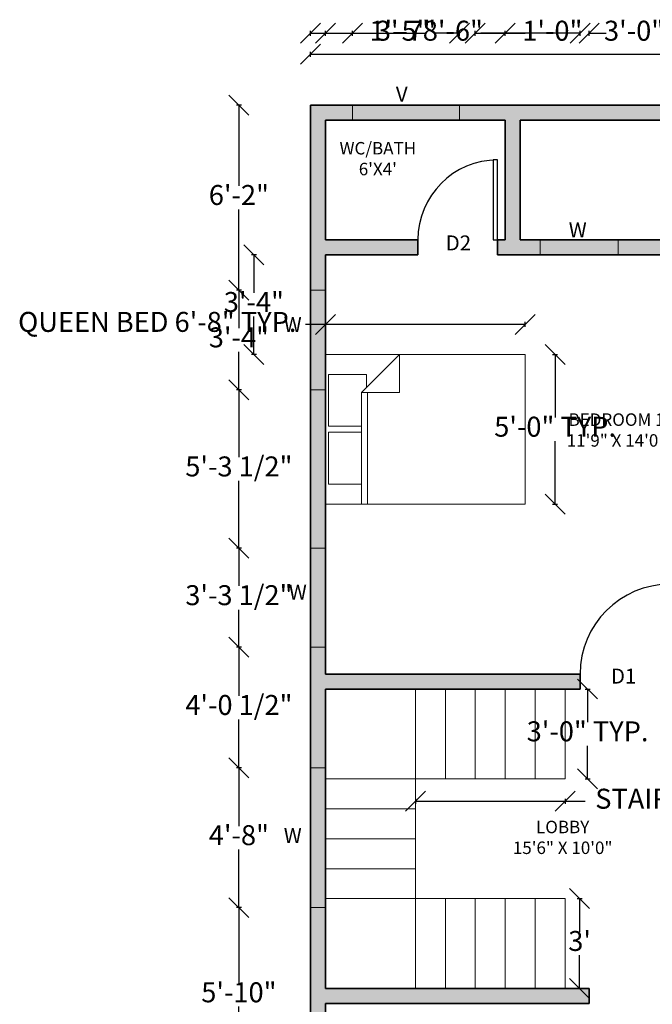
# Model space of a CAD drawing. Units: inches. Extents: x 2247 to 2713, y 588 to 1209.
# Tile 4 of 5: x 2247 to 2501, y 808 to 1202. Entities that reach past the tile are written whole.
import ezdxf

# ---------------------------------------------------------------- set-up
doc = ezdxf.new("R2010")
doc.units = ezdxf.units.IN
for name, color, linetype, lineweight in [('A-ANNO-DIMS', 2, 'Continuous', 18), ('A-ANNO-TEXT', 7, 'Continuous', 18), ('A-AREA-IDEN', 7, 'Continuous', 25), ('A-DOOR', 3, 'Continuous', 25), ('A-FLOR-STRS', 7, 'Continuous', 18), ('A-FURN', 8, 'Continuous', 18), ('A-GLAZ', 4, 'Continuous', 18), ('A-GLAZ-PATT', 7, 'Continuous', 13), ('A-WALL', 7, 'Continuous', 35), ('A-WALL-PATT', 4, 'Continuous', 13)]:
    doc.layers.add(name, color=color, linetype=linetype, lineweight=lineweight)
doc.styles.get("Standard").update_dxf_attribs({"font": 'arial.ttf'})
doc.dimstyles.new('ISO-25', dxfattribs={"dimtxt": 8, "dimasz": 8, "dimexe": 1, "dimexo": 1, "dimtad": 0, "dimtih": 1, "dimtoh": 1, "dimlunit": 3, "dimtxsty": 'Standard', "dimblk": 'OBLIQUE', "dimcen": 2.5, "dimadec": 0, "dimazin": 0, "dimtfac": 1, "dimtmove": 0, "dimatfit": 3, "dimfxl": 1, "dimfxlon": 1, "dimarcsym": 0})

# ---------------------------------------------------------------- blocks, each defined once
blk = doc.blocks.new('*U4')
for p, q in [((0, 0), (0, -6)), ((-36, 0), (-36, -6))]:
    blk.add_line(p, q)
blk.add_lwpolyline([(0, 0), (0, 36), (-1.75, 36), (-1.75, 0)], close=True)
blk.add_arc((0, 0), 36, 90, 180)
blk = doc.blocks.new('*U6')
for p, q in [((0, 0), (0, -6)), ((-32, 0), (-32, -6))]:
    blk.add_line(p, q)
blk.add_lwpolyline([(0, 0), (0, 32), (-1.75, 32), (-1.75, 0)], close=True)
blk.add_arc((0, 0), 32, 90, 180)
blk = doc.blocks.new('Bed - Queen')
for p, q in [((0, -80.00003), (0, 0)), ((0, 0), (59.99999, 0)), ((59.99999, 0), (59.99999, -80.00003)), ((7.99999, -1.2), (28.79998, -1.2)), ((7.99999, -14.4), (7.99999, -1.2)), ((28.79998, -1.2), (28.79998, -14.4)), ((31.19999, -1.2), (51.99999, -1.2)), ((31.19999, -14.4), (31.19999, -1.2)), ((51.99999, -1.2), (51.99999, -16.4)), ((0, -14.4), (44.8, -14.4)), ((59.99999, -29.6), (44.8, -14.4)), ((44.8, -14.4), (44.8, -29.6)), ((44.8, -16.8), (0, -16.8)), ((51.99999, -16.4), (46.79936, -16.4)), ((44.8, -29.6), (59.99999, -29.6)), ((59.99999, -80.00003), (0, -80.00003))]:
    blk.add_line(p, q)
blk = doc.blocks.new('_Oblique')
at = {"color": 0, "linetype": 'ByBlock', "lineweight": -2}
blk.add_line((-0.5, -0.5), (0.5, 0.5), dxfattribs=at)
blk = doc.blocks.new('*D11')
at = {"layer": 'A-ANNO-DIMS', "color": 0, "lineweight": -2, "transparency": 16777216}
for p, q in [((2364.08, 1187.64), (2364.08, 1189.64)), ((2364.08, 1188.64), (2506.59, 1188.64)), ((2664.08, 1188.64), (2521.56, 1188.64)), ((2664.08, 1187.64), (2664.08, 1189.64))]:
    blk.add_line(p, q, dxfattribs=at)
at = {"layer": 'Defpoints', "color": 0, "transparency": 16777216}
for p in [(2664.08, 1188.64), (2364.08, 1168.28), (2664.08, 1168.28)]:
    blk.add_point(p, dxfattribs=at)
at = {"layer": 'A-ANNO-DIMS', "color": 0, "lineweight": -2, "transparency": 16777216, "xscale": 8, "yscale": 8, "zscale": 8, "rotation": 180}
blk.add_blockref('_Oblique', (2364.08, 1188.64), dxfattribs=at)
at = {"layer": 'A-ANNO-DIMS', "color": 0, "lineweight": -2, "transparency": 16777216, "xscale": 8, "yscale": 8, "zscale": 8}
blk.add_blockref('_Oblique', (2664.08, 1188.64), dxfattribs=at)
at = {"layer": 'A-ANNO-DIMS', "color": 0, "transparency": 16777216, "insert": (2514.08, 1188.64), "char_height": 8, "attachment_point": 5}
blk.add_mtext("25'", dxfattribs=at)
blk = doc.blocks.new('*D13')
at = {"layer": 'A-ANNO-DIMS', "color": 0, "lineweight": -2, "transparency": 16777216}
for p, q in [((2470.88, 850.28), (2472.88, 850.28)), ((2471.88, 850.28), (2471.88, 836.99)), ((2471.88, 814.28), (2471.88, 827.57)), ((2470.88, 814.28), (2472.88, 814.28))]:
    blk.add_line(p, q, dxfattribs=at)
at = {"layer": 'Defpoints', "color": 0, "transparency": 16777216}
for p in [(2466.08, 850.28), (2466.08, 814.28), (2471.88, 814.28)]:
    blk.add_point(p, dxfattribs=at)
at = {"layer": 'A-ANNO-DIMS', "color": 0, "lineweight": -2, "transparency": 16777216, "xscale": 8, "yscale": 8, "zscale": 8}
for p, rotation in [((2471.88, 850.28), 90), ((2471.88, 814.28), 270)]:
    blk.add_blockref('_Oblique', p, dxfattribs=dict(at, rotation=rotation))
at = {"layer": 'A-ANNO-DIMS', "color": 0, "transparency": 16777216, "insert": (2471.88, 832.28), "char_height": 8, "attachment_point": 5}
blk.add_mtext("3'", dxfattribs=at)
blk = doc.blocks.new('STAIR-FLIGHT-36IN-12IN-GOING')
for p, q in [((0, 36), (0, 0)), ((12, 36), (12, 0)), ((24, 36), (24, 0)), ((36, 36), (36, 0)), ((48, 36), (48, 0)), ((60, 36), (60, 0))]:
    blk.add_line(p, q)
blk = doc.blocks.new('*D15')
at = {"layer": 'A-ANNO-DIMS', "color": 0, "lineweight": -2, "transparency": 16777216}
for p, q in [((2370.08, 1079.35), (2370.08, 1081.35)), ((2450.08, 1079.35), (2450.08, 1081.35)), ((2370.08, 1080.35), (2362.08, 1080.35)), ((2450.08, 1080.35), (2370.08, 1080.35))]:
    blk.add_line(p, q, dxfattribs=at)
at = {"layer": 'Defpoints', "color": 0, "transparency": 16777216}
for p in [(2370.08, 1080.35), (2370.08, 1068.35), (2450.08, 1068.35)]:
    blk.add_point(p, dxfattribs=at)
at = {"layer": 'A-ANNO-DIMS', "color": 0, "lineweight": -2, "transparency": 16777216, "xscale": 8, "yscale": 8, "zscale": 8, "rotation": 180}
blk.add_blockref('_Oblique', (2370.08, 1080.35), dxfattribs=at)
at = {"layer": 'A-ANNO-DIMS', "color": 0, "lineweight": -2, "transparency": 16777216, "xscale": 8, "yscale": 8, "zscale": 8}
blk.add_blockref('_Oblique', (2450.08, 1080.35), dxfattribs=at)
at = {"layer": 'A-ANNO-DIMS', "color": 0, "transparency": 16777216, "insert": (2302.61, 1080.35), "char_height": 8, "attachment_point": 5}
blk.add_mtext('QUEEN BED 6\'-8" TYP.', dxfattribs=at)
blk = doc.blocks.new('*D16')
at = {"layer": 'A-ANNO-DIMS', "color": 0, "lineweight": -2, "transparency": 16777216}
for p, q in [((2461.08, 1068.35), (2463.08, 1068.35)), ((2462.08, 1068.35), (2462.08, 1043.06)), ((2462.08, 1008.35), (2462.08, 1033.64)), ((2461.08, 1008.35), (2463.08, 1008.35))]:
    blk.add_line(p, q, dxfattribs=at)
at = {"layer": 'Defpoints', "color": 0, "transparency": 16777216}
for p in [(2450.08, 1068.35), (2462.08, 1068.35), (2450.08, 1008.35)]:
    blk.add_point(p, dxfattribs=at)
at = {"layer": 'A-ANNO-DIMS', "color": 0, "lineweight": -2, "transparency": 16777216, "xscale": 8, "yscale": 8, "zscale": 8}
for p, rotation in [((2462.08, 1068.35), 90), ((2462.08, 1008.35), 270)]:
    blk.add_blockref('_Oblique', p, dxfattribs=dict(at, rotation=rotation))
at = {"layer": 'A-ANNO-DIMS', "color": 0, "transparency": 16777216, "insert": (2462.08, 1038.35), "char_height": 8, "attachment_point": 5}
blk.add_mtext('5\'-0" TYP.', dxfattribs=at)
blk = doc.blocks.new('*D17')
at = {"layer": 'A-ANNO-DIMS', "color": 0, "lineweight": -2, "transparency": 16777216}
for p, q in [((2406.08, 890.28), (2406.08, 888.28)), ((2406.08, 889.28), (2466.08, 889.28)), ((2466.08, 890.28), (2466.08, 888.28)), ((2466.08, 889.28), (2474.08, 889.28))]:
    blk.add_line(p, q, dxfattribs=at)
at = {"layer": 'Defpoints', "color": 0, "transparency": 16777216}
for p in [(2406.08, 898.28), (2466.08, 898.28), (2466.08, 889.28)]:
    blk.add_point(p, dxfattribs=at)
at = {"layer": 'A-ANNO-DIMS', "color": 0, "lineweight": -2, "transparency": 16777216, "xscale": 8, "yscale": 8, "zscale": 8, "rotation": 180}
blk.add_blockref('_Oblique', (2406.08, 889.28), dxfattribs=at)
at = {"layer": 'A-ANNO-DIMS', "color": 0, "lineweight": -2, "transparency": 16777216, "xscale": 8, "yscale": 8, "zscale": 8}
blk.add_blockref('_Oblique', (2466.08, 889.28), dxfattribs=at)
at = {"layer": 'A-ANNO-DIMS', "color": 0, "transparency": 16777216, "insert": (2538.49, 889.28), "char_height": 8, "attachment_point": 5}
blk.add_mtext('STAIR FLIGHT 5\'-0" TYP.', dxfattribs=at)
blk = doc.blocks.new('*D18')
at = {"layer": 'A-ANNO-DIMS', "color": 0, "lineweight": -2, "transparency": 16777216}
for p, q in [((2474.08, 934.28), (2476.08, 934.28)), ((2475.08, 934.28), (2475.08, 920.99)), ((2475.08, 898.28), (2475.08, 911.57)), ((2474.08, 898.28), (2476.08, 898.28))]:
    blk.add_line(p, q, dxfattribs=at)
at = {"layer": 'Defpoints', "color": 0, "transparency": 16777216}
for p in [(2466.08, 934.28), (2475.08, 934.28), (2466.08, 898.28)]:
    blk.add_point(p, dxfattribs=at)
at = {"layer": 'A-ANNO-DIMS', "color": 0, "lineweight": -2, "transparency": 16777216, "xscale": 8, "yscale": 8, "zscale": 8}
for p, rotation in [((2475.08, 934.28), 90), ((2475.08, 898.28), 270)]:
    blk.add_blockref('_Oblique', p, dxfattribs=dict(at, rotation=rotation))
at = {"layer": 'A-ANNO-DIMS', "color": 0, "transparency": 16777216, "insert": (2475.08, 916.28), "char_height": 8, "attachment_point": 5}
blk.add_mtext('3\'-0" TYP.', dxfattribs=at)
blk = doc.blocks.new('*D27')
at = {"layer": 'A-ANNO-DIMS', "color": 0, "lineweight": -2, "transparency": 16777216}
for p, q in [((2407.02, 600.53), (2407.02, 598.53)), ((2439.02, 600.53), (2439.02, 598.53)), ((2407.02, 599.53), (2411.7, 599.53)), ((2439.02, 599.53), (2434.35, 599.53))]:
    blk.add_line(p, q, dxfattribs=at)
at = {"layer": 'Defpoints', "color": 0, "transparency": 16777216}
for p in [(2407.02, 1108.28), (2439.02, 1108.28), (2439.02, 599.53)]:
    blk.add_point(p, dxfattribs=at)
at = {"layer": 'A-ANNO-DIMS', "color": 0, "lineweight": -2, "transparency": 16777216, "xscale": 8, "yscale": 8, "zscale": 8, "rotation": 180}
blk.add_blockref('_Oblique', (2407.02, 599.53), dxfattribs=at)
at = {"layer": 'A-ANNO-DIMS', "color": 0, "lineweight": -2, "transparency": 16777216, "xscale": 8, "yscale": 8, "zscale": 8}
blk.add_blockref('_Oblique', (2439.02, 599.53), dxfattribs=at)
at = {"layer": 'A-ANNO-DIMS', "color": 0, "transparency": 16777216, "insert": (2423.02, 599.53), "char_height": 8, "attachment_point": 5}
blk.add_mtext('2\'-8"', dxfattribs=at)
blk = doc.blocks.new('*D29')
at = {"layer": 'A-ANNO-DIMS', "color": 0, "lineweight": -2, "transparency": 16777216}
for p, q in [((2336.33, 1094.13), (2334.33, 1094.13)), ((2335.33, 1094.13), (2335.33, 1078.86)), ((2335.33, 1054.17), (2335.33, 1069.44)), ((2336.33, 1054.17), (2334.33, 1054.17))]:
    blk.add_line(p, q, dxfattribs=at)
at = {"layer": 'Defpoints', "color": 0, "transparency": 16777216}
for p in [(2335.33, 1094.13), (2364.08, 1094.13), (2364.08, 1054.17)]:
    blk.add_point(p, dxfattribs=at)
at = {"layer": 'A-ANNO-DIMS', "color": 0, "lineweight": -2, "transparency": 16777216, "xscale": 8, "yscale": 8, "zscale": 8}
for p, rotation in [((2335.33, 1094.13), 90), ((2335.33, 1054.17), 270)]:
    blk.add_blockref('_Oblique', p, dxfattribs=dict(at, rotation=rotation))
at = {"layer": 'A-ANNO-DIMS', "color": 0, "transparency": 16777216, "insert": (2335.33, 1074.15), "char_height": 8, "attachment_point": 5}
blk.add_mtext('3\'-4"', dxfattribs=at)
blk = doc.blocks.new('*D30')
at = {"layer": 'A-ANNO-DIMS', "color": 0, "lineweight": -2, "transparency": 16777216}
for p, q in [((2336.33, 990.69), (2334.33, 990.69)), ((2335.33, 990.69), (2335.33, 975.6)), ((2335.33, 950.99), (2335.33, 966.07)), ((2336.33, 950.99), (2334.33, 950.99))]:
    blk.add_line(p, q, dxfattribs=at)
at = {"layer": 'Defpoints', "color": 0, "transparency": 16777216}
for p in [(2335.33, 990.69), (2364.08, 990.69), (2364.08, 950.99)]:
    blk.add_point(p, dxfattribs=at)
at = {"layer": 'A-ANNO-DIMS', "color": 0, "lineweight": -2, "transparency": 16777216, "xscale": 8, "yscale": 8, "zscale": 8}
for p, rotation in [((2335.33, 990.69), 90), ((2335.33, 950.99), 270)]:
    blk.add_blockref('_Oblique', p, dxfattribs=dict(at, rotation=rotation))
at = {"layer": 'A-ANNO-DIMS', "color": 0, "transparency": 16777216, "insert": (2335.33, 970.84), "char_height": 8, "attachment_point": 5}
blk.add_mtext('3\'-3 1/2"', dxfattribs=at)
blk = doc.blocks.new('*D31')
at = {"layer": 'A-ANNO-DIMS', "color": 0, "lineweight": -2, "transparency": 16777216}
for p, q in [((2336.33, 1054.17), (2334.33, 1054.17)), ((2335.33, 1054.17), (2335.33, 1027.19)), ((2335.33, 990.69), (2335.33, 1017.67)), ((2336.33, 990.69), (2334.33, 990.69))]:
    blk.add_line(p, q, dxfattribs=at)
at = {"layer": 'Defpoints', "color": 0, "transparency": 16777216}
for p in [(2335.33, 1054.17), (2364.08, 1054.17), (2364.08, 990.69)]:
    blk.add_point(p, dxfattribs=at)
at = {"layer": 'A-ANNO-DIMS', "color": 0, "lineweight": -2, "transparency": 16777216, "xscale": 8, "yscale": 8, "zscale": 8}
for p, rotation in [((2335.33, 1054.17), 90), ((2335.33, 990.69), 270)]:
    blk.add_blockref('_Oblique', p, dxfattribs=dict(at, rotation=rotation))
at = {"layer": 'A-ANNO-DIMS', "color": 0, "transparency": 16777216, "insert": (2335.33, 1022.43), "char_height": 8, "attachment_point": 5}
blk.add_mtext('5\'-3 1/2"', dxfattribs=at)
blk = doc.blocks.new('*D32')
at = {"layer": 'A-ANNO-DIMS', "color": 0, "lineweight": -2, "transparency": 16777216}
for p, q in [((2336.33, 1168.28), (2334.33, 1168.28)), ((2335.33, 1168.28), (2335.33, 1135.91)), ((2335.33, 1094.13), (2335.33, 1126.49)), ((2336.33, 1094.13), (2334.33, 1094.13))]:
    blk.add_line(p, q, dxfattribs=at)
at = {"layer": 'Defpoints', "color": 0, "transparency": 16777216}
for p in [(2335.33, 1168.28), (2364.08, 1168.28), (2364.08, 1094.13)]:
    blk.add_point(p, dxfattribs=at)
at = {"layer": 'A-ANNO-DIMS', "color": 0, "lineweight": -2, "transparency": 16777216, "xscale": 8, "yscale": 8, "zscale": 8}
for p, rotation in [((2335.33, 1168.28), 90), ((2335.33, 1094.13), 270)]:
    blk.add_blockref('_Oblique', p, dxfattribs=dict(at, rotation=rotation))
at = {"layer": 'A-ANNO-DIMS', "color": 0, "transparency": 16777216, "insert": (2335.33, 1131.2), "char_height": 8, "attachment_point": 5}
blk.add_mtext('6\'-2"', dxfattribs=at)
blk = doc.blocks.new('*D35')
at = {"layer": 'A-ANNO-DIMS', "color": 0, "lineweight": -2, "transparency": 16777216}
for p, q in [((2336.33, 846.66), (2334.33, 846.66)), ((2335.33, 846.66), (2335.33, 816.41)), ((2335.33, 776.75), (2335.33, 806.99)), ((2336.33, 776.75), (2334.33, 776.75))]:
    blk.add_line(p, q, dxfattribs=at)
at = {"layer": 'Defpoints', "color": 0, "transparency": 16777216}
for p in [(2335.33, 846.66), (2364.08, 846.66), (2364.08, 776.75)]:
    blk.add_point(p, dxfattribs=at)
at = {"layer": 'A-ANNO-DIMS', "color": 0, "lineweight": -2, "transparency": 16777216, "xscale": 8, "yscale": 8, "zscale": 8}
for p, rotation in [((2335.33, 846.66), 90), ((2335.33, 776.75), 270)]:
    blk.add_blockref('_Oblique', p, dxfattribs=dict(at, rotation=rotation))
at = {"layer": 'A-ANNO-DIMS', "color": 0, "transparency": 16777216, "insert": (2335.33, 811.7), "char_height": 8, "attachment_point": 5}
blk.add_mtext('5\'-10"', dxfattribs=at)
blk = doc.blocks.new('*D36')
at = {"layer": 'A-ANNO-DIMS', "color": 0, "lineweight": -2, "transparency": 16777216}
for p, q in [((2336.33, 902.69), (2334.33, 902.69)), ((2335.33, 902.69), (2335.33, 879.38)), ((2335.33, 846.66), (2335.33, 869.97)), ((2336.33, 846.66), (2334.33, 846.66))]:
    blk.add_line(p, q, dxfattribs=at)
at = {"layer": 'Defpoints', "color": 0, "transparency": 16777216}
for p in [(2335.33, 902.69), (2364.08, 902.69), (2364.08, 846.66)]:
    blk.add_point(p, dxfattribs=at)
at = {"layer": 'A-ANNO-DIMS', "color": 0, "lineweight": -2, "transparency": 16777216, "xscale": 8, "yscale": 8, "zscale": 8}
for p, rotation in [((2335.33, 902.69), 90), ((2335.33, 846.66), 270)]:
    blk.add_blockref('_Oblique', p, dxfattribs=dict(at, rotation=rotation))
at = {"layer": 'A-ANNO-DIMS', "color": 0, "transparency": 16777216, "insert": (2335.33, 874.67), "char_height": 8, "attachment_point": 5}
blk.add_mtext('4\'-8"', dxfattribs=at)
blk = doc.blocks.new('*D37')
at = {"layer": 'A-ANNO-DIMS', "color": 0, "lineweight": -2, "transparency": 16777216}
for p, q in [((2336.33, 950.99), (2334.33, 950.99)), ((2335.33, 950.99), (2335.33, 931.6)), ((2335.33, 902.69), (2335.33, 922.08)), ((2336.33, 902.69), (2334.33, 902.69))]:
    blk.add_line(p, q, dxfattribs=at)
at = {"layer": 'Defpoints', "color": 0, "transparency": 16777216}
for p in [(2335.33, 950.99), (2364.08, 950.99), (2364.08, 902.69)]:
    blk.add_point(p, dxfattribs=at)
at = {"layer": 'A-ANNO-DIMS', "color": 0, "lineweight": -2, "transparency": 16777216, "xscale": 8, "yscale": 8, "zscale": 8}
for p, rotation in [((2335.33, 950.99), 90), ((2335.33, 902.69), 270)]:
    blk.add_blockref('_Oblique', p, dxfattribs=dict(at, rotation=rotation))
at = {"layer": 'A-ANNO-DIMS', "color": 0, "transparency": 16777216, "insert": (2335.33, 926.84), "char_height": 8, "attachment_point": 5}
blk.add_mtext('4\'-0 1/2"', dxfattribs=at)
blk = doc.blocks.new('*D41')
at = {"layer": 'A-ANNO-DIMS', "color": 0, "lineweight": -2, "transparency": 16777216}
for p, q in [((2380.83, 1196.03), (2380.83, 1198.03)), ((2380.83, 1197.03), (2391.02, 1197.03)), ((2423.72, 1197.03), (2413.53, 1197.03)), ((2423.72, 1196.03), (2423.72, 1198.03))]:
    blk.add_line(p, q, dxfattribs=at)
at = {"layer": 'Defpoints', "color": 0, "transparency": 16777216}
for p in [(2423.72, 1197.03), (2380.83, 1168.28), (2423.72, 1168.28)]:
    blk.add_point(p, dxfattribs=at)
at = {"layer": 'A-ANNO-DIMS', "color": 0, "lineweight": -2, "transparency": 16777216, "xscale": 8, "yscale": 8, "zscale": 8, "rotation": 180}
blk.add_blockref('_Oblique', (2380.83, 1197.03), dxfattribs=at)
at = {"layer": 'A-ANNO-DIMS', "color": 0, "lineweight": -2, "transparency": 16777216, "xscale": 8, "yscale": 8, "zscale": 8}
blk.add_blockref('_Oblique', (2423.72, 1197.03), dxfattribs=at)
at = {"layer": 'A-ANNO-DIMS', "color": 0, "transparency": 16777216, "insert": (2402.27, 1197.03), "char_height": 8, "attachment_point": 5}
blk.add_mtext('3\'-7"', dxfattribs=at)
blk = doc.blocks.new('*D43')
at = {"layer": 'A-ANNO-DIMS', "color": 0, "lineweight": -2, "transparency": 16777216}
for p, q in [((2364.08, 1196.03), (2364.08, 1198.03)), ((2364.08, 1197.03), (2380.83, 1197.03)), ((2380.83, 1196.03), (2380.83, 1198.03)), ((2380.83, 1197.03), (2388.83, 1197.03))]:
    blk.add_line(p, q, dxfattribs=at)
at = {"layer": 'Defpoints', "color": 0, "transparency": 16777216}
for p in [(2380.83, 1197.03), (2364.08, 1168.28), (2380.83, 1168.28)]:
    blk.add_point(p, dxfattribs=at)
at = {"layer": 'A-ANNO-DIMS', "color": 0, "lineweight": -2, "transparency": 16777216, "xscale": 8, "yscale": 8, "zscale": 8, "rotation": 180}
blk.add_blockref('_Oblique', (2364.08, 1197.03), dxfattribs=at)
at = {"layer": 'A-ANNO-DIMS', "color": 0, "lineweight": -2, "transparency": 16777216, "xscale": 8, "yscale": 8, "zscale": 8}
blk.add_blockref('_Oblique', (2380.83, 1197.03), dxfattribs=at)
at = {"layer": 'A-ANNO-DIMS', "color": 0, "transparency": 16777216, "insert": (2399.71, 1197.03), "char_height": 8, "attachment_point": 5}
blk.add_mtext('1\'-5"', dxfattribs=at)
blk = doc.blocks.new('*D45')
at = {"layer": 'A-ANNO-DIMS', "color": 0, "lineweight": -2, "transparency": 16777216}
for p, q in [((2456.06, 600.53), (2456.06, 598.53)), ((2487.37, 600.53), (2487.37, 598.53)), ((2456.06, 599.53), (2487.37, 599.53)), ((2487.37, 599.53), (2495.37, 599.53))]:
    blk.add_line(p, q, dxfattribs=at)
at = {"layer": 'Defpoints', "color": 0, "transparency": 16777216}
for p in [(2456.06, 1108.28), (2487.37, 1108.28), (2487.37, 599.53)]:
    blk.add_point(p, dxfattribs=at)
at = {"layer": 'A-ANNO-DIMS', "color": 0, "lineweight": -2, "transparency": 16777216, "xscale": 8, "yscale": 8, "zscale": 8, "rotation": 180}
blk.add_blockref('_Oblique', (2456.06, 599.53), dxfattribs=at)
at = {"layer": 'A-ANNO-DIMS', "color": 0, "lineweight": -2, "transparency": 16777216, "xscale": 8, "yscale": 8, "zscale": 8}
blk.add_blockref('_Oblique', (2487.37, 599.53), dxfattribs=at)
at = {"layer": 'A-ANNO-DIMS', "color": 0, "transparency": 16777216, "insert": (2516.02, 599.53), "char_height": 8, "attachment_point": 5}
blk.add_mtext('2\'-7 1/2"', dxfattribs=at)
blk = doc.blocks.new('*D47')
at = {"layer": 'A-ANNO-DIMS', "color": 0, "lineweight": -2, "transparency": 16777216}
for p, q in [((2487.37, 600.53), (2487.37, 598.53)), ((2524.66, 600.53), (2524.66, 598.53)), ((2487.37, 599.53), (2524.66, 599.53)), ((2524.66, 599.53), (2532.66, 599.53))]:
    blk.add_line(p, q, dxfattribs=at)
at = {"layer": 'Defpoints', "color": 0, "transparency": 16777216}
for p in [(2487.37, 1108.28), (2524.66, 1108.28), (2524.66, 599.53)]:
    blk.add_point(p, dxfattribs=at)
at = {"layer": 'A-ANNO-DIMS', "color": 0, "lineweight": -2, "transparency": 16777216, "xscale": 8, "yscale": 8, "zscale": 8, "rotation": 180}
blk.add_blockref('_Oblique', (2487.37, 599.53), dxfattribs=at)
at = {"layer": 'A-ANNO-DIMS', "color": 0, "lineweight": -2, "transparency": 16777216, "xscale": 8, "yscale": 8, "zscale": 8}
blk.add_blockref('_Oblique', (2524.66, 599.53), dxfattribs=at)
at = {"layer": 'A-ANNO-DIMS', "color": 0, "transparency": 16777216, "insert": (2553.24, 599.53), "char_height": 8, "attachment_point": 5}
blk.add_mtext('3\'-1 1/2"', dxfattribs=at)
blk = doc.blocks.new('*D48')
at = {"layer": 'A-ANNO-DIMS', "color": 0, "lineweight": -2, "transparency": 16777216}
for p, q in [((2448.08, 600.53), (2448.08, 598.53)), ((2456.06, 600.53), (2456.06, 598.53)), ((2448.08, 599.53), (2440.08, 599.53)), ((2456.06, 599.53), (2448.08, 599.53))]:
    blk.add_line(p, q, dxfattribs=at)
at = {"layer": 'Defpoints', "color": 0, "transparency": 16777216}
for p in [(2448.08, 1114.28), (2456.06, 1114.28), (2448.08, 599.53)]:
    blk.add_point(p, dxfattribs=at)
at = {"layer": 'A-ANNO-DIMS', "color": 0, "lineweight": -2, "transparency": 16777216, "xscale": 8, "yscale": 8, "zscale": 8, "rotation": 180}
blk.add_blockref('_Oblique', (2448.08, 599.53), dxfattribs=at)
at = {"layer": 'A-ANNO-DIMS', "color": 0, "lineweight": -2, "transparency": 16777216, "xscale": 8, "yscale": 8, "zscale": 8}
blk.add_blockref('_Oblique', (2456.06, 599.53), dxfattribs=at)
at = {"layer": 'A-ANNO-DIMS', "color": 0, "transparency": 16777216, "insert": (2428.82, 599.53), "char_height": 8, "attachment_point": 5}
blk.add_mtext('0\'-8"', dxfattribs=at)
blk = doc.blocks.new('*D54')
at = {"layer": 'A-ANNO-DIMS', "color": 0, "lineweight": -2, "transparency": 16777216}
for p, q in [((2430.08, 1196.03), (2430.08, 1198.03)), ((2430.08, 1197.03), (2442.08, 1197.03)), ((2442.08, 1196.03), (2442.08, 1198.03)), ((2442.08, 1197.03), (2450.08, 1197.03))]:
    blk.add_line(p, q, dxfattribs=at)
at = {"layer": 'Defpoints', "color": 0, "transparency": 16777216}
for p in [(2442.08, 1197.03), (2430.08, 850.28), (2442.08, 850.28)]:
    blk.add_point(p, dxfattribs=at)
at = {"layer": 'A-ANNO-DIMS', "color": 0, "lineweight": -2, "transparency": 16777216, "xscale": 8, "yscale": 8, "zscale": 8, "rotation": 180}
blk.add_blockref('_Oblique', (2430.08, 1197.03), dxfattribs=at)
at = {"layer": 'A-ANNO-DIMS', "color": 0, "lineweight": -2, "transparency": 16777216, "xscale": 8, "yscale": 8, "zscale": 8}
blk.add_blockref('_Oblique', (2442.08, 1197.03), dxfattribs=at)
at = {"layer": 'A-ANNO-DIMS', "color": 0, "transparency": 16777216, "insert": (2460.96, 1197.03), "char_height": 8, "attachment_point": 5}
blk.add_mtext('1\'-0"', dxfattribs=at)
blk = doc.blocks.new('*D55')
at = {"layer": 'A-ANNO-DIMS', "color": 0, "lineweight": -2, "transparency": 16777216}
for p, q in [((2439.02, 600.53), (2439.02, 598.53)), ((2442.08, 600.53), (2442.08, 598.53)), ((2439.02, 599.53), (2442.08, 599.53)), ((2442.08, 599.53), (2450.08, 599.53))]:
    blk.add_line(p, q, dxfattribs=at)
at = {"layer": 'Defpoints', "color": 0, "transparency": 16777216}
for p in [(2442.08, 1114.28), (2439.02, 1108.28), (2442.08, 599.53)]:
    blk.add_point(p, dxfattribs=at)
at = {"layer": 'A-ANNO-DIMS', "color": 0, "lineweight": -2, "transparency": 16777216, "xscale": 8, "yscale": 8, "zscale": 8, "rotation": 180}
blk.add_blockref('_Oblique', (2439.02, 599.53), dxfattribs=at)
at = {"layer": 'A-ANNO-DIMS', "color": 0, "lineweight": -2, "transparency": 16777216, "xscale": 8, "yscale": 8, "zscale": 8}
blk.add_blockref('_Oblique', (2442.08, 599.53), dxfattribs=at)
at = {"layer": 'A-ANNO-DIMS', "color": 0, "transparency": 16777216, "insert": (2461.33, 599.53), "char_height": 8, "attachment_point": 5}
blk.add_mtext('0\'-3"', dxfattribs=at)
blk = doc.blocks.new('*D56')
at = {"layer": 'A-ANNO-DIMS', "color": 0, "lineweight": -2, "transparency": 16777216}
for p, q in [((2370.08, 1196.03), (2370.08, 1198.03)), ((2370.08, 1197.03), (2409.81, 1197.03)), ((2472.08, 1197.03), (2432.34, 1197.03)), ((2472.08, 1196.03), (2472.08, 1198.03))]:
    blk.add_line(p, q, dxfattribs=at)
at = {"layer": 'Defpoints', "color": 0, "transparency": 16777216}
for p in [(2370.08, 1197.03), (2370.08, 940.28), (2472.08, 940.28)]:
    blk.add_point(p, dxfattribs=at)
at = {"layer": 'A-ANNO-DIMS', "color": 0, "lineweight": -2, "transparency": 16777216, "xscale": 8, "yscale": 8, "zscale": 8, "rotation": 180}
blk.add_blockref('_Oblique', (2370.08, 1197.03), dxfattribs=at)
at = {"layer": 'A-ANNO-DIMS', "color": 0, "lineweight": -2, "transparency": 16777216, "xscale": 8, "yscale": 8, "zscale": 8}
blk.add_blockref('_Oblique', (2472.08, 1197.03), dxfattribs=at)
at = {"layer": 'A-ANNO-DIMS', "color": 0, "transparency": 16777216, "insert": (2421.08, 1197.03), "char_height": 8, "attachment_point": 5}
blk.add_mtext('8\'-6"', dxfattribs=at)
blk = doc.blocks.new('*D58')
at = {"layer": 'A-ANNO-DIMS', "color": 0, "lineweight": -2, "transparency": 16777216}
for p, q in [((2475.72, 1196.03), (2475.72, 1198.03)), ((2475.72, 1197.03), (2482.47, 1197.03)), ((2511.72, 1197.03), (2504.98, 1197.03)), ((2511.72, 1196.03), (2511.72, 1198.03))]:
    blk.add_line(p, q, dxfattribs=at)
at = {"layer": 'Defpoints', "color": 0, "transparency": 16777216}
for p in [(2511.72, 1197.03), (2475.72, 814.28), (2511.72, 814.28)]:
    blk.add_point(p, dxfattribs=at)
at = {"layer": 'A-ANNO-DIMS', "color": 0, "lineweight": -2, "transparency": 16777216, "xscale": 8, "yscale": 8, "zscale": 8, "rotation": 180}
blk.add_blockref('_Oblique', (2475.72, 1197.03), dxfattribs=at)
at = {"layer": 'A-ANNO-DIMS', "color": 0, "lineweight": -2, "transparency": 16777216, "xscale": 8, "yscale": 8, "zscale": 8}
blk.add_blockref('_Oblique', (2511.72, 1197.03), dxfattribs=at)
at = {"layer": 'A-ANNO-DIMS', "color": 0, "transparency": 16777216, "insert": (2493.72, 1197.03), "char_height": 8, "attachment_point": 5}
blk.add_mtext('3\'-0"', dxfattribs=at)
blk = doc.blocks.new('*D60')
at = {"layer": 'A-ANNO-DIMS', "color": 0, "lineweight": -2, "transparency": 16777216}
for p, q in [((2342.33, 1108.28), (2340.33, 1108.28)), ((2341.33, 1108.28), (2341.33, 1093.03)), ((2341.33, 1068.35), (2341.33, 1083.6)), ((2342.33, 1068.35), (2340.33, 1068.35))]:
    blk.add_line(p, q, dxfattribs=at)
at = {"layer": 'Defpoints', "color": 0, "transparency": 16777216}
for p in [(2341.33, 1108.28), (2370.08, 1108.28), (2370.08, 1068.35)]:
    blk.add_point(p, dxfattribs=at)
at = {"layer": 'A-ANNO-DIMS', "color": 0, "lineweight": -2, "transparency": 16777216, "xscale": 8, "yscale": 8, "zscale": 8}
for p, rotation in [((2341.33, 1108.28), 90), ((2341.33, 1068.35), 270)]:
    blk.add_blockref('_Oblique', p, dxfattribs=dict(at, rotation=rotation))
at = {"layer": 'A-ANNO-DIMS', "color": 0, "transparency": 16777216, "insert": (2341.33, 1088.32), "char_height": 8, "attachment_point": 5}
blk.add_mtext('3\'-4"', dxfattribs=at)

msp = doc.modelspace()

# ---------------------------------------------------------------- hatches: boundary and pattern name
at = {"layer": 'A-GLAZ-PATT'}
h = msp.add_hatch(color=256, dxfattribs=at)
h.dxf.hatch_style = 1
h.paths.add_polyline_path([(2423.716, 1168.28), (2380.833, 1168.28), (2380.833, 1162.28), (2423.716, 1162.28)])
h.paths.add_polyline_path([(2487.371, 1114.28), (2456.056, 1114.28), (2456.056, 1108.28), (2487.371, 1108.28)])
h.paths.add_polyline_path([(2560.507, 1114.28), (2524.66, 1114.28), (2524.66, 1108.28), (2560.507, 1108.28)])
h.paths.add_polyline_path([(2639.393, 1168.28), (2604.041, 1168.28), (2604.041, 1162.28), (2639.393, 1162.28)])
h.paths.add_polyline_path([(2370.076, 1094.128), (2364.076, 1094.128), (2364.076, 1054.172), (2370.076, 1054.172), (2370.076, 1068.35)])
h.paths.add_polyline_path([(2370.076, 990.686), (2364.076, 990.686), (2364.076, 950.99), (2370.076, 950.99)])
h.paths.add_polyline_path([(2664.076, 1094.128), (2658.076, 1094.128), (2658.076, 1054.172), (2664.076, 1054.172)])
h.paths.add_polyline_path([(2664.076, 990.686), (2658.076, 990.686), (2658.076, 950.99), (2664.076, 950.99)])
h.paths.add_polyline_path([(2664.076, 913.24), (2658.076, 913.24), (2658.076, 861.585), (2664.076, 861.585)])
h.paths.add_polyline_path([(2626.201, 814.28), (2584.934, 814.28), (2584.934, 808.28), (2626.201, 808.28)])
h.paths.add_polyline_path([(2370.076, 902.687), (2364.076, 902.687), (2364.076, 846.663), (2370.076, 846.663)])
h.paths.add_polyline_path([(2370.076, 776.746), (2364.076, 776.746), (2364.076, 709.673), (2370.076, 709.673)])
h.paths.add_polyline_path([(2457.582, 679.28), (2410.479, 679.28), (2410.479, 673.28), (2457.582, 673.28)])
at = {"layer": 'A-WALL-PATT'}
h = msp.add_hatch(color=256, dxfattribs=at)
h.dxf.hatch_style = 1
h.paths.add_polyline_path([(2604.041, 1168.28), (2423.716, 1168.28), (2423.716, 1162.28), (2442.076, 1162.28), (2442.076, 1114.28), (2439.021, 1114.28), (2439.021, 1108.28), (2456.056, 1108.28), (2456.056, 1114.28), (2448.076, 1114.28), (2448.076, 1162.28), (2580.076, 1162.28), (2580.076, 1114.28), (2560.507, 1114.28), (2560.507, 1108.28), (2619.195, 1108.28), (2619.195, 1114.28), (2586.076, 1114.28), (2586.076, 1162.28), (2604.041, 1162.28)])
h.paths.add_polyline_path([(2380.833, 1168.28), (2364.076, 1168.28), (2364.076, 1094.128), (2370.076, 1094.128), (2370.076, 1108.28), (2407.021, 1108.28), (2407.021, 1114.28), (2370.076, 1114.28), (2370.076, 1162.28), (2380.833, 1162.28)])
h.paths.add_polyline_path([(2664.076, 1168.28), (2639.393, 1168.28), (2639.393, 1162.28), (2658.076, 1162.28), (2658.076, 1114.28), (2651.195, 1114.28), (2651.195, 1108.28), (2658.076, 1108.28), (2658.076, 1094.128), (2664.076, 1094.128)])
h.paths.add_polyline_path([(2524.66, 1114.28), (2487.371, 1114.28), (2487.371, 1108.28), (2511.076, 1108.28), (2511.076, 940.28), (2508.076, 940.28), (2508.076, 934.28), (2520.076, 934.28), (2520.076, 940.28), (2517.076, 940.28), (2517.076, 1108.28), (2524.66, 1108.28)])
h.paths.add_polyline_path([(2370.076, 1054.172), (2364.076, 1054.172), (2364.076, 990.686), (2370.076, 990.686)])
h.paths.add_polyline_path([(2370.076, 934.28), (2472.076, 934.28), (2472.076, 940.28), (2370.076, 940.28), (2370.076, 950.99), (2364.076, 950.99), (2364.076, 902.687), (2370.076, 902.687)])
h.paths.add_polyline_path([(2664.076, 950.99), (2658.076, 950.99), (2658.076, 940.28), (2556.076, 940.28), (2556.076, 934.28), (2658.076, 934.28), (2658.076, 913.24), (2664.076, 913.24)])
h.paths.add_polyline_path([(2664.076, 1054.172), (2658.076, 1054.172), (2658.076, 990.686), (2664.076, 990.686)])
h.paths.add_polyline_path([(2664.076, 861.585), (2658.076, 861.585), (2658.076, 814.28), (2626.201, 814.28), (2626.201, 808.28), (2658.076, 808.28), (2658.076, 628.28), (2664.076, 628.28)])
h.paths.add_polyline_path([(2562.076, 871.28), (2556.076, 871.28), (2556.076, 808.28), (2584.934, 808.28), (2584.934, 814.28), (2562.076, 814.28)])
h.paths.add_polyline_path([(2475.722, 808.28), (2370.076, 808.28), (2370.076, 776.746), (2364.076, 776.746), (2364.076, 846.663), (2370.076, 846.663), (2370.076, 814.28), (2475.722, 814.28)])
h.paths.add_polyline_path([(2370.076, 709.673), (2364.076, 709.673), (2364.076, 628.28), (2520.076, 628.28), (2520.076, 634.28), (2370.076, 634.28)])
h.paths.add_polyline_path([(2410.479, 679.28), (2370.076, 679.28), (2370.076, 673.28), (2410.479, 673.28)], flags=17)
h.paths.add_polyline_path([(2520.076, 679.28), (2514.076, 679.28), (2474.076, 679.28), (2457.582, 679.28), (2457.582, 673.28), (2520.076, 673.28)], flags=17)
h.paths.add_polyline_path([(2520.076, 814.28), (2511.722, 814.28), (2511.722, 808.28), (2514.076, 808.28), (2514.076, 719.28), (2520.076, 719.28)])

# ---------------------------------------------------------------- linework, layer by layer
at = {"layer": 'A-FLOR-STRS'}
for p, q in [((2466.076, 898.28), (2370.076, 898.28)), ((2406.076, 898.28), (2406.076, 850.28)), ((2406.076, 886.28), (2370.076, 886.28)), ((2406.076, 874.28), (2370.076, 874.28)), ((2406.076, 862.28), (2370.076, 862.28)), ((2406.076, 850.28), (2370.076, 850.28)), ((2466.076, 850.28), (2406.076, 850.28))]:
    msp.add_line(p, q, dxfattribs=at)
at = {"layer": 'A-GLAZ'}
for p, q in [((2380.833, 1162.28), (2380.833, 1168.28)), ((2423.716, 1162.28), (2423.716, 1168.28)), ((2456.056, 1114.28), (2456.056, 1108.28)), ((2487.371, 1114.28), (2487.371, 1108.28)), ((2370.076, 1094.128), (2364.076, 1094.128)), ((2364.076, 1054.172), (2370.076, 1054.172)), ((2364.076, 990.686), (2370.076, 990.686)), ((2370.076, 950.99), (2364.076, 950.99)), ((2370.076, 902.687), (2364.076, 902.687)), ((2369.634, 846.663), (2364.076, 846.663))]:
    msp.add_line(p, q, dxfattribs=at)
at = {"layer": 'A-WALL'}
for p, q in [((2664.076, 1168.28), (2364.076, 1168.28)), ((2364.076, 1168.28), (2364.076, 628.28)), ((2370.076, 1162.28), (2370.076, 1114.28)), ((2442.076, 1162.28), (2370.076, 1162.28)), ((2442.076, 1162.28), (2442.076, 1114.28)), ((2448.076, 1162.28), (2448.076, 1114.28)), ((2580.076, 1162.28), (2448.076, 1162.28)), ((2407.021, 1114.28), (2370.076, 1114.28)), ((2407.021, 1114.28), (2407.021, 1108.28)), ((2442.076, 1114.28), (2439.021, 1114.28)), ((2439.021, 1114.28), (2439.021, 1108.28)), ((2580.076, 1114.28), (2448.076, 1114.28)), ((2370.076, 1108.28), (2370.076, 940.28)), ((2407.021, 1108.28), (2370.076, 1108.28)), ((2511.076, 1108.28), (2439.021, 1108.28)), ((2472.076, 940.28), (2370.076, 940.28)), ((2472.076, 940.28), (2472.076, 934.28)), ((2370.076, 934.28), (2370.076, 814.28)), ((2472.076, 934.28), (2370.076, 934.28)), ((2475.722, 814.28), (2370.076, 814.28)), ((2475.722, 808.28), (2475.722, 814.28)), ((2370.076, 808.28), (2370.076, 679.28)), ((2475.722, 808.28), (2370.076, 808.28))]:
    msp.add_line(p, q, dxfattribs=at)

# ---------------------------------------------------------------- block references
at = {"layer": 'A-DOOR'}
for name, p in [('*U6', (2439.021, 1114.28)), ('*U4', (2508.076, 940.28))]:
    msp.add_blockref(name, p, dxfattribs=at)
at = {"layer": 'A-FLOR-STRS'}
msp.add_blockref('STAIR-FLIGHT-36IN-12IN-GOING', (2406.076, 898.28), dxfattribs=at)
at = {"layer": 'A-FLOR-STRS', "rotation": 180}
msp.add_blockref('STAIR-FLIGHT-36IN-12IN-GOING', (2466.076, 850.28), dxfattribs=at)
at = {"layer": 'A-FURN', "rotation": 90}
msp.add_blockref('Bed - Queen', (2370.076, 1008.35), dxfattribs=at)

# ---------------------------------------------------------------- texts
at = {"layer": 'A-ANNO-TEXT', "char_height": 6, "attachment_point": 1}
for s, insert in [('\\pxqc;V', (2394.654, 1175.618)), ('\\pxqc;W', (2465.177, 1121.232)), ('\\pxqc;D2', (2417.35, 1116.031)), ('\\pxqc;W', (2350.96, 1083.367)), ('\\pxqc;W', (2353.002, 976.086)), ('\\pxqc;D1', (2483.583, 942.458)), ('\\pxqc;W', (2350.96, 878.562))]:
    msp.add_mtext_dynamic_manual_height_columns(s, width=11.90357, gutter_width=12.5, heights=[0], dxfattribs=dict(at, insert=insert))
at = {"layer": 'A-AREA-IDEN', "char_height": 5, "attachment_point": 1}
for s, width, insert in [("\\pxqc;WC/BATH\\P6'X4'", 33.16994, (2374.433, 1153.469)), ('\\pxqc;BEDROOM 1\\P11\'9" X 14\'0"', 45.05776, (2464.156, 1044.727)), ('\\pxqc;LOBBY\\P15\'6" X 10\'0"', 49.7829, (2440.202, 881.491))]:
    msp.add_mtext_dynamic_manual_height_columns(s, width=width, gutter_width=12.5, heights=[0], dxfattribs=dict(at, insert=insert))

# ---------------------------------------------------------------- dimensions: what is measured, and where the dimension line sits
at = {"layer": 'A-ANNO-DIMS'}
for base, p1, p2, override, picture, middle in [((2380.833, 1197.03), (2364.076, 1168.28), (2380.833, 1168.28), {"dimdec": 1, "dimlfac": 1, "dimrnd": 0, "dimzin": 1, "dimdsep": 46, "dimlunit": 4, "dimfrac": 2}, '*D43', (2399.714, 1197.03)), ((2370.076, 1197.03), (2472.076, 940.28), (2370.076, 940.28), {"dimdec": 1, "dimlfac": 1, "dimrnd": 0, "dimzin": 1, "dimdsep": 46, "dimlunit": 4, "dimfrac": 2}, '*D56', (2421.076, 1197.03)), ((2423.716, 1197.03), (2380.833, 1168.28), (2423.716, 1168.28), {"dimdec": 1, "dimlfac": 1, "dimrnd": 0, "dimzin": 1, "dimdsep": 46, "dimlunit": 4, "dimfrac": 2}, '*D41', (2402.275, 1197.03)), ((2442.076, 1197.03), (2430.076, 850.28), (2442.076, 850.28), {"dimdec": 1, "dimlfac": 1, "dimrnd": 0, "dimzin": 1, "dimdsep": 46, "dimlunit": 4, "dimfrac": 2}, '*D54', (2460.957, 1197.03)), ((2511.722, 1197.03), (2475.722, 814.28), (2511.722, 814.28), {"dimdec": 1, "dimlfac": 1, "dimrnd": 0, "dimzin": 1, "dimdsep": 46, "dimlunit": 4, "dimfrac": 2}, '*D58', (2493.722, 1197.03)), ((2664.076, 1188.641), (2364.076, 1168.28), (2664.076, 1168.28), {"dimclrd": 0, "dimclre": 0, "dimclrt": 0}, '*D11', (2514.076, 1188.641)), ((2448.076, 599.53), (2456.056, 1114.28), (2448.076, 1114.28), {"dimdec": 1, "dimlfac": 1, "dimrnd": 0, "dimzin": 1, "dimdsep": 46, "dimlunit": 4, "dimfrac": 2}, '*D48', (2428.818, 599.53)), ((2442.076, 599.53), (2439.021, 1108.28), (2442.076, 1114.28), {"dimdec": 1, "dimlfac": 1, "dimrnd": 0, "dimzin": 1, "dimdsep": 46, "dimlunit": 4, "dimfrac": 2}, '*D55', (2461.334, 599.53)), ((2439.021, 599.53), (2407.021, 1108.28), (2439.021, 1108.28), {"dimdec": 1, "dimlfac": 1, "dimrnd": 0, "dimzin": 1, "dimdsep": 46, "dimlunit": 4, "dimfrac": 2}, '*D27', (2423.021, 599.53)), ((2487.371, 599.53), (2456.056, 1108.28), (2487.371, 1108.28), {"dimdec": 1, "dimlfac": 1, "dimrnd": 0, "dimzin": 1, "dimdsep": 46, "dimlunit": 4, "dimfrac": 2}, '*D45', (2516.018, 599.53)), ((2524.66, 599.53), (2487.371, 1108.28), (2524.66, 1108.28), {"dimdec": 1, "dimlfac": 1, "dimrnd": 0, "dimzin": 1, "dimdsep": 46, "dimlunit": 4, "dimfrac": 2}, '*D47', (2553.236, 599.53))]:
    dim = msp.add_linear_dim(base=base, p1=p1, p2=p2, dimstyle='ISO-25', override=override, dxfattribs=at)
    dim.commit()
    dim.dimension.update_dxf_attribs({"geometry": picture, "text_midpoint": middle})
for base, p1, p2, override, picture, middle in [((2335.326, 1168.28), (2364.076, 1094.128), (2364.076, 1168.28), {"dimdec": 1, "dimlfac": 1, "dimrnd": 0, "dimzin": 1, "dimdsep": 46, "dimlunit": 4, "dimfrac": 2}, '*D32', (2335.326, 1131.204)), ((2341.326, 1108.28), (2370.076, 1068.35), (2370.076, 1108.28), {"dimdec": 1, "dimlfac": 1, "dimrnd": 0, "dimzin": 1, "dimdsep": 46, "dimlunit": 4, "dimfrac": 2}, '*D60', (2341.326, 1088.315)), ((2335.326, 1094.128), (2364.076, 1054.172), (2364.076, 1094.128), {"dimdec": 1, "dimlfac": 1, "dimrnd": 0, "dimzin": 1, "dimdsep": 46, "dimlunit": 4, "dimfrac": 2}, '*D29', (2335.326, 1074.15)), ((2335.326, 1054.172), (2364.076, 990.686), (2364.076, 1054.172), {"dimdec": 1, "dimlfac": 1, "dimrnd": 0, "dimzin": 1, "dimdsep": 46, "dimlunit": 4, "dimfrac": 2}, '*D31', (2335.326, 1022.429)), ((2335.326, 990.686), (2364.076, 950.99), (2364.076, 990.686), {"dimdec": 1, "dimlfac": 1, "dimrnd": 0, "dimzin": 1, "dimdsep": 46, "dimlunit": 4, "dimfrac": 2}, '*D30', (2335.326, 970.838)), ((2335.326, 950.99), (2364.076, 902.687), (2364.076, 950.99), {"dimdec": 1, "dimlfac": 1, "dimrnd": 0, "dimzin": 1, "dimdsep": 46, "dimlunit": 4, "dimfrac": 2}, '*D37', (2335.326, 926.839)), ((2335.326, 902.687), (2364.076, 846.663), (2364.076, 902.687), {"dimdec": 1, "dimlfac": 1, "dimrnd": 0, "dimzin": 1, "dimdsep": 46, "dimlunit": 4, "dimfrac": 2}, '*D36', (2335.326, 874.675)), ((2471.882, 814.28), (2466.076, 850.28), (2466.076, 814.28), {"dimclrd": 0, "dimclre": 0, "dimclrt": 0}, '*D13', (2471.882, 832.28)), ((2335.326, 846.663), (2364.076, 776.746), (2364.076, 846.663), {"dimdec": 1, "dimlfac": 1, "dimrnd": 0, "dimzin": 1, "dimdsep": 46, "dimlunit": 4, "dimfrac": 2}, '*D35', (2335.326, 811.704))]:
    dim = msp.add_linear_dim(base=base, p1=p1, p2=p2, angle=90, dimstyle='ISO-25', override=override, dxfattribs=at)
    dim.commit()
    dim.dimension.update_dxf_attribs({"geometry": picture, "text_midpoint": middle})
for base, p1, p2, angle, text, picture, middle in [((2370.076, 1080.35), (2450.076, 1068.35), (2370.076, 1068.35), 180, 'QUEEN BED <> TYP.', '*D15', (2302.611, 1080.35)), ((2462.076, 1068.35), (2450.076, 1008.35), (2450.076, 1068.35), 90, '<> TYP.', '*D16', (2462.076, 1038.35)), ((2475.076, 934.28), (2466.076, 898.28), (2466.076, 934.28), 90, '<> TYP.', '*D18', (2475.076, 916.28))]:
    dim = msp.add_linear_dim(base=base, p1=p1, p2=p2, angle=angle, text=text, dimstyle='ISO-25', override={"dimdec": 1, "dimlfac": 1, "dimrnd": 0, "dimzin": 1, "dimdsep": 46, "dimlunit": 4, "dimfrac": 2}, dxfattribs=at)
    dim.commit()
    dim.dimension.update_dxf_attribs({"geometry": picture, "text_midpoint": middle})
dim = msp.add_linear_dim(base=(2466.076, 889.28), p1=(2406.076, 898.28), p2=(2466.076, 898.28), text='STAIR FLIGHT <> TYP.', dimstyle='ISO-25', override={"dimdec": 1, "dimlfac": 1, "dimrnd": 0, "dimzin": 1, "dimdsep": 46, "dimlunit": 4, "dimfrac": 2}, dxfattribs=at)
dim.commit()
dim.dimension.update_dxf_attribs({"geometry": '*D17', "text_midpoint": (2538.494, 889.28)})

doc.saveas('drawing.dxf')
